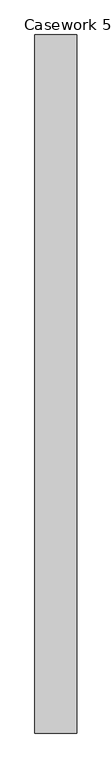
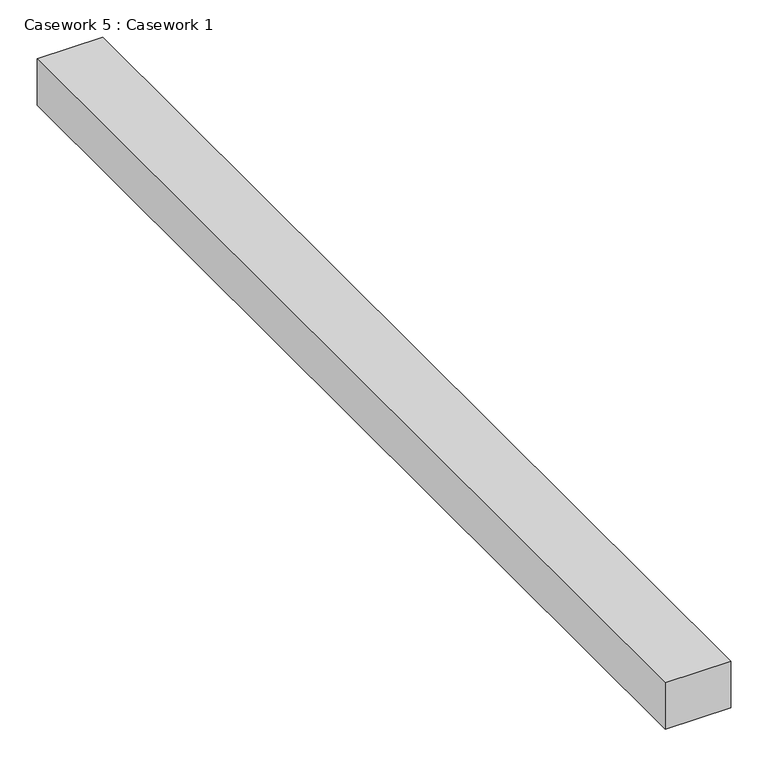
"""IFC4 building model written with IfcOpenShell, lengths in millimetres: furniture geometry, Casework 5 : Casework 1."""

from ifc_helpers import new_model, si_unit, frame, origin, place, context, project, spatial, polyline, outline, extrude, source, transform, mapped, element, save


def casework_5_casework_1_a4356d40(model_context):
    return source(origin(), model_context, "Body", "SweptSolid", [
        extrude(outline(polyline([(8443.3559589, 14787.9496924), (8443.3559589, 13098.8496924), (8341.7559589, 13098.8496924), (8341.7559589, 14787.9496924), (8443.3559589, 14787.9496924)])), frame((0.0, 0.0, 3581.4), z_axis=(0.0, 0.0, 1.0), x_axis=(1.0, 0.0, 0.0)), (0.0, 0.0, 1.0), 76.2),
    ])


if __name__ == "__main__":
    model = new_model("IFC4")
    model_context = context("Model", 3, world=origin())
    ifc_project = project(units=[si_unit("LENGTHUNIT", "METRE", prefix="MILLI")], contexts=[model_context])
    site = spatial("IfcSite", under=ifc_project)
    building = spatial("IfcBuilding", under=site)
    placement = place(None, origin())
    casework_5_casework_1_shape = casework_5_casework_1_a4356d40(model_context)
    element("IfcFurniture", 1, ObjectType="Casework 5 : Casework 1", at=placement, inside=building, context=model_context, shape_type="MappedRepresentation", body=[
        mapped(casework_5_casework_1_shape, transform((0.0, 0.0, 0.0), x_axis=(1.0, 0.0, 0.0), y_axis=(0.0, 1.0, 0.0), z_axis=(0.0, 0.0, 1.0))),
    ])
    save(model, "model.ifc")

# Revit data of these elements
# Element 1 (IfcFurniture, "Casework 5 : Casework 1")
#   Materials on its faces: "Clad - White"
# Materials
#   "Clad - White": class "Wood", colour RGB 242 242 238, transparency 0, Cost = 0
